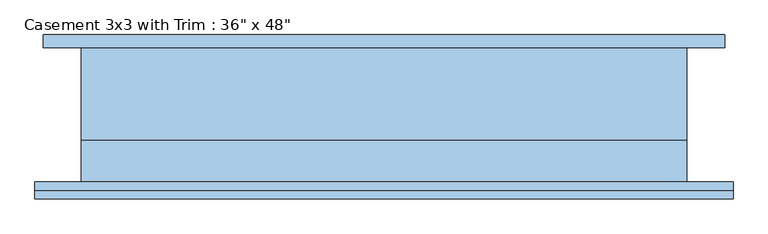
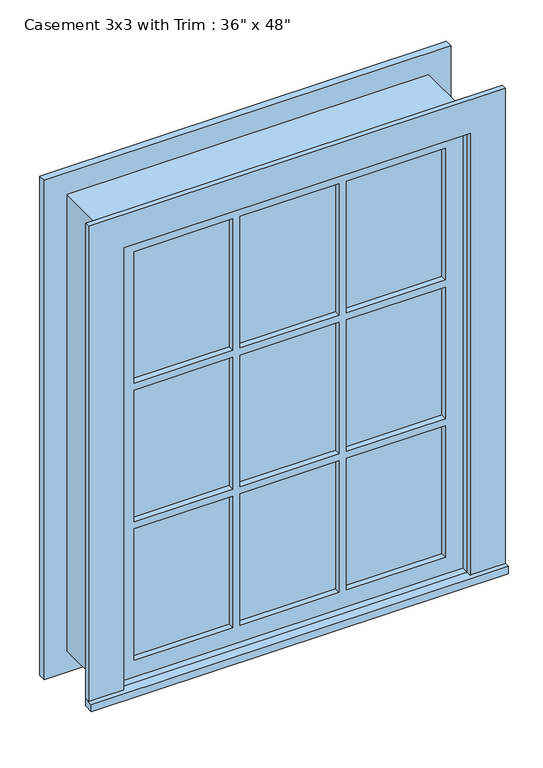
"""IFC4 building model written with IfcOpenShell, lengths in millimetres: window geometry."""

from ifc_helpers import new_model, si_unit, frame, origin, place, context, project, spatial, polyline, outline, extrude, source, transform, mapped, element, save


def window_ce5e1bf6(model_context):
    return source(origin(), model_context, "Body", "SweptSolid", [
        extrude(outline(polyline([(-527.05, -127.0), (-527.05, -101.6), (527.05, -101.6), (527.05, -127.0), (-527.05, -127.0)])), frame((0.0, 0.0, 914.4), z_axis=(0.0, 0.0, 1.0), x_axis=(1.0, 0.0, 0.0)), (0.0, 0.0, 1.0), 19.05),
        extrude(outline(polyline([(2114.55, -438.15), (2114.55, 438.15), (933.45, 438.15), (933.45, 527.05), (2203.45, 527.05), (2203.45, -527.05), (933.45, -527.05), (933.45, -438.15), (2114.55, -438.15)])), frame((0.0, -114.3, 0.0), z_axis=(0.0, 1.0, 0.0), x_axis=(0.0, 0.0, 1.0)), (0.0, 0.0, 1.0), 12.7),
        extrude(outline(polyline([(143.9333333, -66.675), (143.9333333, -53.975), (393.7, -53.975), (393.7, -66.675), (143.9333333, -66.675)])), frame((0.0, 0.0, 1718.7333333), z_axis=(0.0, 0.0, 1.0), x_axis=(1.0, 0.0, 0.0)), (0.0, 0.0, 1.0), 351.3666667),
        extrude(outline(polyline([(-124.8833333, -66.675), (-124.8833333, -53.975), (124.8833333, -53.975), (124.8833333, -66.675), (-124.8833333, -66.675)])), frame((0.0, 0.0, 1718.7333333), z_axis=(0.0, 0.0, 1.0), x_axis=(1.0, 0.0, 0.0)), (0.0, 0.0, 1.0), 351.3666667),
        extrude(outline(polyline([(-393.7, -66.675), (-393.7, -53.975), (-143.9333333, -53.975), (-143.9333333, -66.675), (-393.7, -66.675)])), frame((0.0, 0.0, 1718.7333333), z_axis=(0.0, 0.0, 1.0), x_axis=(1.0, 0.0, 0.0)), (0.0, 0.0, 1.0), 351.3666667),
        extrude(outline(polyline([(-393.7, -66.675), (-393.7, -53.975), (-143.9333333, -53.975), (-143.9333333, -66.675), (-393.7, -66.675)])), frame((0.0, 0.0, 1348.3166667), z_axis=(0.0, 0.0, 1.0), x_axis=(1.0, 0.0, 0.0)), (0.0, 0.0, 1.0), 351.3666667),
        extrude(outline(polyline([(-124.8833333, -66.675), (-124.8833333, -53.975), (124.8833333, -53.975), (124.8833333, -66.675), (-124.8833333, -66.675)])), frame((0.0, 0.0, 1348.3166667), z_axis=(0.0, 0.0, 1.0), x_axis=(1.0, 0.0, 0.0)), (0.0, 0.0, 1.0), 351.3666667),
        extrude(outline(polyline([(143.9333333, -66.675), (143.9333333, -53.975), (393.7, -53.975), (393.7, -66.675), (143.9333333, -66.675)])), frame((0.0, 0.0, 1348.3166667), z_axis=(0.0, 0.0, 1.0), x_axis=(1.0, 0.0, 0.0)), (0.0, 0.0, 1.0), 351.3666667),
        extrude(outline(polyline([(143.9333333, -66.675), (143.9333333, -53.975), (393.7, -53.975), (393.7, -66.675), (143.9333333, -66.675)])), frame((0.0, 0.0, 977.9), z_axis=(0.0, 0.0, 1.0), x_axis=(1.0, 0.0, 0.0)), (0.0, 0.0, 1.0), 351.3666667),
        extrude(outline(polyline([(-124.8833333, -66.675), (-124.8833333, -53.975), (124.8833333, -53.975), (124.8833333, -66.675), (-124.8833333, -66.675)])), frame((0.0, 0.0, 977.9), z_axis=(0.0, 0.0, 1.0), x_axis=(1.0, 0.0, 0.0)), (0.0, 0.0, 1.0), 351.3666667),
        extrude(outline(polyline([(-393.7, -66.675), (-393.7, -53.975), (-143.9333333, -53.975), (-143.9333333, -66.675), (-393.7, -66.675)])), frame((0.0, 0.0, 977.9), z_axis=(0.0, 0.0, 1.0), x_axis=(1.0, 0.0, 0.0)), (0.0, 0.0, 1.0), 351.3666667),
        extrude(outline(polyline([(2190.75, 514.35), (2190.75, -514.35), (857.25, -514.35), (857.25, 514.35), (2190.75, 514.35)]), holes=[polyline([(2101.85, 425.45), (946.15, 425.45), (946.15, -425.45), (2101.85, -425.45), (2101.85, 425.45)])]), frame((0.0, 101.6, 0.0), z_axis=(0.0, 1.0, 0.0), x_axis=(0.0, 0.0, 1.0)), (0.0, 0.0, 1.0), 19.05),
        extrude(outline(polyline([(2114.55, -438.15), (933.45, -438.15), (933.45, 438.15), (2114.55, 438.15), (2114.55, -438.15)]), holes=[polyline([(2070.1, -143.9333333), (1718.7333333, -143.9333333), (1718.7333333, -393.7), (2070.1, -393.7), (2070.1, -143.9333333)]), polyline([(1699.6833333, -143.9333333), (1348.3166667, -143.9333333), (1348.3166667, -393.7), (1699.6833333, -393.7), (1699.6833333, -143.9333333)]), polyline([(1329.2666667, -143.9333333), (977.9, -143.9333333), (977.9, -393.7), (1329.2666667, -393.7), (1329.2666667, -143.9333333)]), polyline([(2070.1, 124.8833333), (1718.7333333, 124.8833333), (1718.7333333, -124.8833333), (2070.1, -124.8833333), (2070.1, 124.8833333)]), polyline([(1699.6833333, 124.8833333), (1348.3166667, 124.8833333), (1348.3166667, -124.8833333), (1699.6833333, -124.8833333), (1699.6833333, 124.8833333)]), polyline([(1329.2666667, 124.8833333), (977.9, 124.8833333), (977.9, -124.8833333), (1329.2666667, -124.8833333), (1329.2666667, 124.8833333)]), polyline([(2070.1, 393.7), (1718.7333333, 393.7), (1718.7333333, 143.9333333), (2070.1, 143.9333333), (2070.1, 393.7)]), polyline([(1699.6833333, 393.7), (1348.3166667, 393.7), (1348.3166667, 143.9333333), (1699.6833333, 143.9333333), (1699.6833333, 393.7)]), polyline([(1329.2666667, 393.7), (977.9, 393.7), (977.9, 143.9333333), (1329.2666667, 143.9333333), (1329.2666667, 393.7)])]), frame((0.0, -82.55, 0.0), z_axis=(0.0, 1.0, 0.0), x_axis=(0.0, 0.0, 1.0)), (0.0, 0.0, 1.0), 44.45),
        extrude(outline(polyline([(2133.6, -457.2), (914.4, -457.2), (914.4, 457.2), (2133.6, 457.2), (2133.6, -457.2)]), holes=[polyline([(2101.85, -425.45), (2101.85, 425.45), (946.15, 425.45), (946.15, -425.45), (2101.85, -425.45)])]), frame((0.0, -38.1, 0.0), z_axis=(0.0, 1.0, 0.0), x_axis=(0.0, 0.0, 1.0)), (0.0, 0.0, 1.0), 139.7),
        extrude(outline(polyline([(2133.6, 457.2), (2133.6, -457.2), (914.4, -457.2), (914.4, 457.2), (2133.6, 457.2)]), holes=[polyline([(2114.55, 438.15), (933.45, 438.15), (933.45, -438.15), (2114.55, -438.15), (2114.55, 438.15)])]), frame((0.0, -101.6, 0.0), z_axis=(0.0, 1.0, 0.0), x_axis=(0.0, 0.0, 1.0)), (0.0, 0.0, 1.0), 63.5),
    ])


if __name__ == "__main__":
    model = new_model("IFC4")
    model_context = context("Model", 3, world=origin())
    ifc_project = project(units=[si_unit("LENGTHUNIT", "METRE", prefix="MILLI")], contexts=[model_context])
    site = spatial("IfcSite", under=ifc_project)
    building = spatial("IfcBuilding", under=site)
    placement = place(None, origin())
    window_shape = window_ce5e1bf6(model_context)
    element("IfcWindow", 1, ObjectType="Casement 3x3 with Trim : 36\" x 48\"", at=placement, inside=building, context=model_context, shape_type="MappedRepresentation", body=[
        mapped(window_shape, transform((0.0, 0.0, 0.0), x_axis=(1.0, 0.0, 0.0), y_axis=(0.0, 1.0, 0.0), z_axis=(0.0, 0.0, 1.0))),
    ])
    save(model, "model.ifc")

# Revit data of these elements
# Type "Casement 3x3 with Trim : 36\" x 48\""
#   Type Mark = "10"
#   Construction Type Id = "GSP4R"
#   Assembly Code = "B2020100"
#   Analytic Construction = "1/8 in Pilkington single glazing"
#   Visual Light Transmittance = 0.9
#   Solar Heat Gain Coefficient = 0.78
#   Heat Transfer Coefficient (U) = 0.6496 BTU/(h·ft²·°F)
#   Height = 4' - 0"
#   Default Sill Height = 3' - 0"
#   Trim Projection - Ext. = 0' - 0 1/2"
#   Trim Projection - Int. = 0' - 0 3/4"
#   Trim Width - Exterior = 0' - 3 1/2"
#   Trim Width - Interior = 0' - 3 1/2"
#   Width = 3' - 0"
#   Window Inset = 0' - 0 3/4"
#   Define Thermal Properties by = 1
#   Glass Pane Material = Glass
#   Sash Material = Sash
#   Trim Exterior Material = Trim
#   Trim Interior Material = Trim
#   Wall Closure = (empty or 0)
# Element 1 (IfcWindow, "Casement 3x3 with Trim : 36\" x 48\"")
#   Materials on its faces: "Sash", "Glass", "Trim"
# Materials
#   "Glass": class "Glass", colour RGB 0 128 192, transparency 0.75, Description = "Soda Lime Glass", Cost = 0
#   "Sash": class "Wood", colour RGB 224 178 126, transparency 0
#   "Trim": class "Wood", colour RGB 224 178 126, transparency 0
